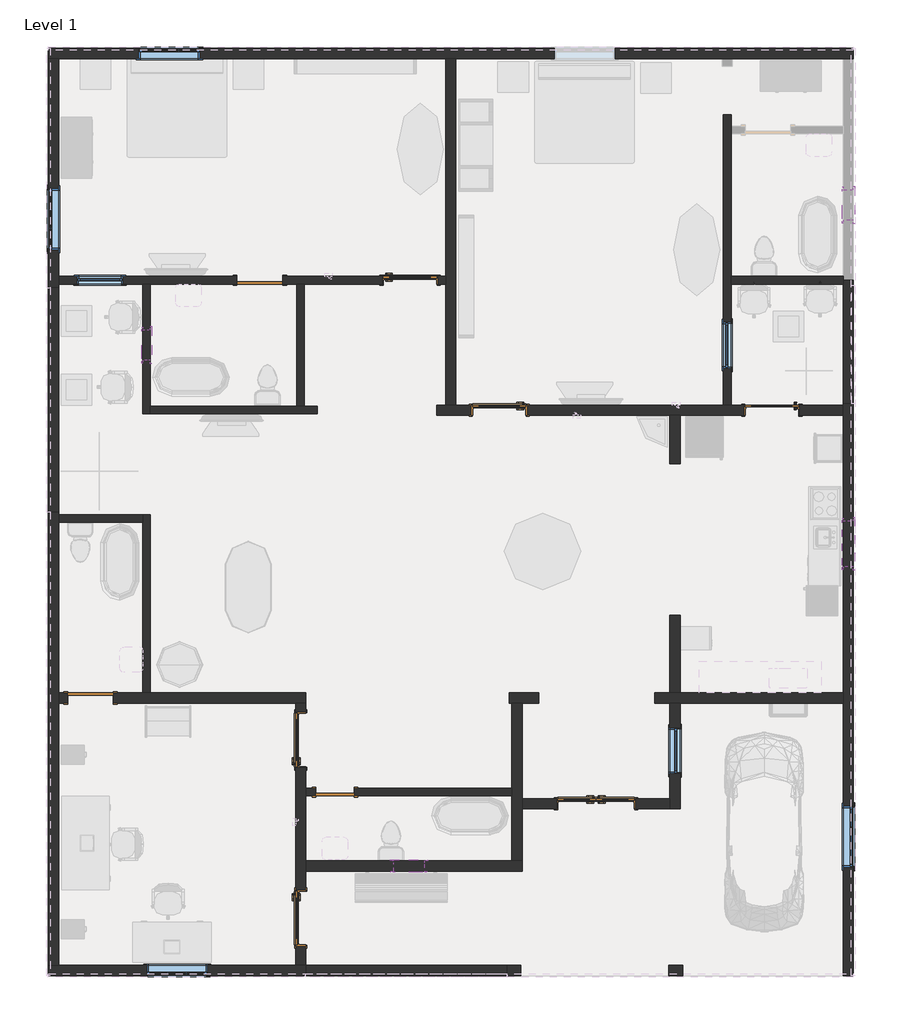
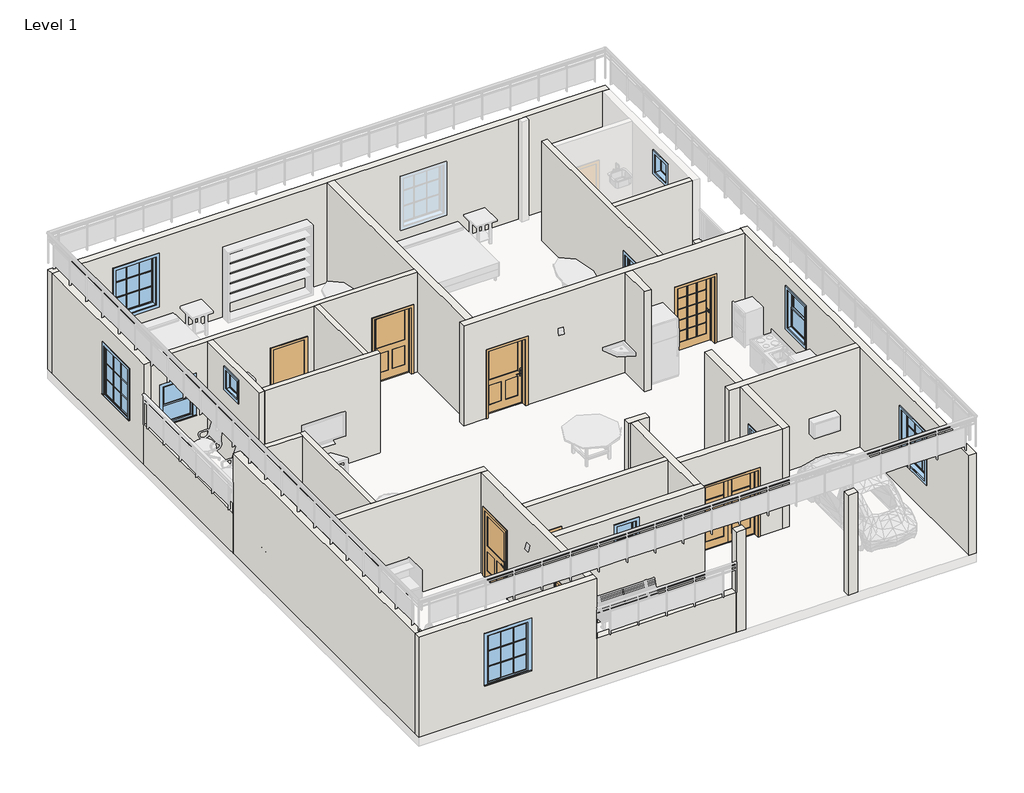
# One storey, part 1 of 4: 31 walls, 11 windows, 9 doors.
"""IFC4 building model written with IfcOpenShell, lengths in millimetres."""

from ifc_helpers import new_model, si_unit, frame, origin, origin_with_axes, place, context, project, spatial, polyline, outline, extrude, faceted_brep, transform, mapped, element, save
from components import door_374e07cf, door_e0076512, door_f970b2d0, door_b03bd389, door_1d83da25, door_059fdd7e, door_719f80de, door_686f89d2, window_cfa1ffdd, window_31198920, window_d24d93a6, window_3d781103, window_e41d21a6

model = new_model("IFC4")

# Units and contexts
model_context = context("Model", 3, world=origin())
ifc_project = project(units=[si_unit("LENGTHUNIT", "METRE", prefix="MILLI")], contexts=[model_context])

# Site, building, storey
site = spatial("IfcSite", under=ifc_project)
building = spatial("IfcBuilding", under=site)
storey = spatial("IfcBuildingStorey", under=building, Name="Level 1", Elevation=0.0)

# Doors
placement = place(None, origin())
door_shape = door_374e07cf(model_context)
element("IfcDoor", 1, ObjectType="42\" x 80\"", at=placement, inside=storey, context=model_context, shape_type="MappedRepresentation", body=[
    mapped(door_shape, transform((-12615.7234731, -1219.5557719, 0.0), x_axis=(0.0, -1.0, 0.0), y_axis=(1.0, 0.0, 0.0), z_axis=(0.0, 0.0, 1.0))),
])
door_2_shape = door_e0076512(model_context)
element("IfcDoor", 2, ObjectType="42\" x 80\"", at=placement, inside=storey, context=model_context, shape_type="MappedRepresentation", body=[
    mapped(door_2_shape, transform((-12615.7234731, -4775.5557719, 0.0), x_axis=(0.0, 1.0, 0.0), y_axis=(-1.0, 0.0, 0.0), z_axis=(0.0, 0.0, 1.0))),
])
element("IfcDoor", 3, ObjectType="42\" x 80\"", at=placement, inside=storey, context=model_context, shape_type="MappedRepresentation", body=[
    mapped(door_2_shape, transform((-8650.1484731, 5362.2192281, 0.0), x_axis=(1.0, 0.0, 0.0), y_axis=(0.0, 1.0, 0.0), z_axis=(0.0, 0.0, 1.0))),
])
door_3_shape = door_f970b2d0(model_context)
element("IfcDoor", 4, ObjectType="42\" x 80\"", at=placement, inside=storey, context=model_context, shape_type="MappedRepresentation", body=[
    mapped(door_3_shape, transform((-10428.1484731, 7953.0192281, 0.0), x_axis=(-1.0, 0.0, 0.0), y_axis=(0.0, -1.0, 0.0), z_axis=(0.0, 0.0, 1.0))),
])
door_4_shape = door_b03bd389(model_context)
element("IfcDoor", 5, ObjectType="Door-Exterior-Double-Full Glass-Wood_Clad : 60\" x 80\"", at=placement, inside=storey, context=model_context, shape_type="MappedRepresentation", body=[
    mapped(door_4_shape, transform((-6719.7484731, -2486.3807719, 0.0), x_axis=(1.0, 0.0, 0.0), y_axis=(0.0, 1.0, 0.0), z_axis=(0.0, 0.0, 1.0))),
])
door_5_shape = door_1d83da25(model_context)
element("IfcDoor", 6, ObjectType="Door-Interior-Single-Full Glass-Wood : 42\" x 80\"", at=placement, inside=storey, context=model_context, shape_type="MappedRepresentation", body=[
    mapped(door_5_shape, transform((-3214.5484731, 5362.2192281, 0.0), x_axis=(-1.0, 0.0, 0.0), y_axis=(0.0, -1.0, 0.0), z_axis=(0.0, 0.0, 1.0))),
])
door_6_shape = door_059fdd7e(model_context)
element("IfcDoor", 7, ObjectType="Single-Flush : 30\" x 80\"", at=placement, inside=storey, context=model_context, shape_type="MappedRepresentation", body=[
    mapped(door_6_shape, transform((-11926.7484731, -2260.9557719, 0.0), x_axis=(-1.0, 0.0, 0.0), y_axis=(0.0, -1.0, 0.0), z_axis=(0.0, 0.0, 1.0))),
])
door_7_shape = door_719f80de(model_context)
element("IfcDoor", 8, ObjectType="Single-Flush : 36\" x 84\"", at=placement, inside=storey, context=model_context, shape_type="MappedRepresentation", body=[
    mapped(door_7_shape, transform((-16803.5484731, -381.3557719, 0.0), x_axis=(-1.0, 0.0, 0.0), y_axis=(0.0, -1.0, 0.0), z_axis=(0.0, 0.0, 1.0))),
])
door_8_shape = door_686f89d2(model_context)
element("IfcDoor", 9, ObjectType="Single-Flush : 36\" x 84\"", at=placement, inside=storey, context=model_context, shape_type="MappedRepresentation", body=[
    mapped(door_8_shape, transform((-13425.3484731, 7949.8442281, 0.0), x_axis=(1.0, 0.0, 0.0), y_axis=(0.0, 1.0, 0.0), z_axis=(0.0, 0.0, 1.0))),
])

# Walls
element("IfcWall", 10, ObjectType="Generic - 8\"", at=placement, inside=storey, context=model_context, shape_type="Brep", body=[
    faceted_brep([(-17641.7484731, 12369.4442281, 0.0), (-17438.5484731, 12369.4442281, 0.0), (-9716.9484731, 12369.4442281, 0.0), (-9513.7484731, 12369.4442281, 0.0), (-4205.1484731, 12369.4442281, 0.0), (-4001.9484731, 12369.4442281, 0.0), (-1792.1484731, 12369.4442281, 0.0), (-1588.9484731, 12369.4442281, 0.0), (-1588.9484731, 12369.4442281, 3048.0), (-1792.1484731, 12369.4442281, 3048.0), (-4001.9484731, 12369.4442281, 3048.0), (-4205.1484731, 12369.4442281, 3048.0), (-9513.7484731, 12369.4442281, 3048.0), (-9716.9484731, 12369.4442281, 3048.0), (-17438.5484731, 12369.4442281, 3048.0), (-17641.7484731, 12369.4442281, 3048.0), (-14619.1484731, 12369.4442281, 2540.0), (-14619.1484731, 12369.4442281, 1016.0), (-15838.3484731, 12369.4442281, 1016.0), (-15838.3484731, 12369.4442281, 2540.0), (-6338.7484731, 12369.4442281, 2438.4), (-6338.7484731, 12369.4442281, 914.4), (-7557.9484731, 12369.4442281, 914.4), (-7557.9484731, 12369.4442281, 2438.4), (-17641.7484731, 12572.6442281, 0.0), (-17641.7484731, 12572.6442281, 3048.0), (-1588.9484731, 12572.6442281, 3048.0), (-1588.9484731, 12572.6442281, 0.0), (-14619.1484731, 12572.6442281, 2540.0), (-15838.3484731, 12572.6442281, 2540.0), (-15838.3484731, 12572.6442281, 1016.0), (-14619.1484731, 12572.6442281, 1016.0), (-6338.7484731, 12572.6442281, 2438.4), (-7557.9484731, 12572.6442281, 2438.4), (-7557.9484731, 12572.6442281, 914.4), (-6338.7484731, 12572.6442281, 914.4)], [[[0, 1, 2, 3, 4, 5, 6, 7, 8, 9, 10, 11, 12, 13, 14, 15], [16, 17, 18, 19], [20, 21, 22, 23]], [[24, 25, 26, 27], [28, 29, 30, 31], [32, 33, 34, 35]], [[7, 6, 5, 4, 3, 2, 1, 0, 24, 27]], [[8, 7, 27, 26]], [[0, 15, 25, 24]], [[17, 16, 28, 31]], [[18, 17, 31, 30]], [[19, 18, 30, 29]], [[16, 19, 29, 28]], [[21, 20, 32, 35]], [[22, 21, 35, 34]], [[23, 22, 34, 33]], [[20, 23, 33, 32]], [[15, 14, 13, 12, 11, 10, 9, 8, 26, 25]]]),
])
element("IfcWall", 11, ObjectType="Generic - 8\"", at=placement, inside=storey, context=model_context, shape_type="Brep", body=[
    faceted_brep([(-17438.5484731, -5715.3557719, 0.0), (-17438.5484731, -482.9557719, 0.0), (-17438.5484731, -279.7557719, 0.0), (-17438.5484731, 3123.8442281, 0.0), (-17438.5484731, 3276.2442281, 0.0), (-17438.5484731, 3327.0442281, 0.0), (-17438.5484731, 3327.0442281, 1219.2), (-17438.5484731, 3327.0442281, 3048.0), (-17438.5484731, 3276.2442281, 3048.0), (-17438.5484731, 3123.8442281, 3048.0), (-17438.5484731, -279.7557719, 3048.0), (-17438.5484731, -482.9557719, 3048.0), (-17438.5484731, -5715.3557719, 3048.0), (-17641.7484731, -5715.3557719, 0.0), (-17641.7484731, -5715.3557719, 3048.0), (-17641.7484731, 3327.0442281, 3048.0), (-17641.7484731, 3327.0442281, 1219.2), (-17641.7484731, 3327.0442281, 0.0)], [[[0, 1, 2, 3, 4, 5, 6, 7, 8, 9, 10, 11, 12]], [[13, 14, 15, 16, 17]], [[5, 4, 3, 2, 1, 0, 13, 17]], [[7, 6, 5, 17, 16, 15]], [[0, 12, 14, 13]], [[12, 11, 10, 9, 8, 7, 15, 14]]]),
])
element("IfcWall", 12, ObjectType="Generic - 8\"", at=placement, inside=storey, context=model_context, shape_type="Brep", body=[
    faceted_brep([(-9716.9484731, 12369.4442281, 0.0), (-9716.9484731, 8026.0442281, 0.0), (-9716.9484731, 7873.6442281, 0.0), (-9716.9484731, 5460.6442281, 0.0), (-9716.9484731, 5460.6442281, 3048.0), (-9716.9484731, 7873.6442281, 3048.0), (-9716.9484731, 8026.0442281, 3048.0), (-9716.9484731, 12369.4442281, 3048.0), (-9513.7484731, 12369.4442281, 0.0), (-9513.7484731, 12369.4442281, 3048.0), (-9513.7484731, 5460.6442281, 3048.0), (-9513.7484731, 5460.6442281, 0.0)], [[[0, 1, 2, 3, 4, 5, 6, 7]], [[8, 9, 10, 11]], [[3, 2, 1, 0, 8, 11]], [[0, 7, 9, 8]], [[4, 3, 11, 10]], [[7, 6, 5, 4, 10, 9]]]),
])
element("IfcWall", 13, ObjectType="Generic - 8\"", at=placement, inside=storey, context=model_context, shape_type="Brep", body=[
    faceted_brep([(-1792.1484731, -279.7557719, 0.0), (-5043.3484731, -279.7557719, 0.0), (-5246.5484731, -279.7557719, 0.0), (-5551.3484731, -279.7557719, 0.0), (-5551.3484731, -279.7557719, 3048.0), (-5246.5484731, -279.7557719, 3048.0), (-5043.3484731, -279.7557719, 3048.0), (-1792.1484731, -279.7557719, 3048.0), (-1792.1484731, -482.9557719, 0.0), (-1792.1484731, -482.9557719, 3048.0), (-5043.3484731, -482.9557719, 3048.0), (-5246.5484731, -482.9557719, 3048.0), (-5551.3484731, -482.9557719, 3048.0), (-5551.3484731, -482.9557719, 0.0), (-5246.5484731, -482.9557719, 0.0), (-5043.3484731, -482.9557719, 0.0)], [[[0, 1, 2, 3, 4, 5, 6, 7]], [[8, 9, 10, 11, 12, 13, 14, 15]], [[3, 2, 1, 0, 8, 15, 14, 13]], [[4, 3, 13, 12]], [[0, 7, 9, 8]], [[7, 6, 5, 4, 12, 11, 10, 9]]]),
])
element("IfcWall", 14, ObjectType="Generic - 8\"", at=placement, inside=storey, context=model_context, shape_type="Brep", body=[
    faceted_brep([(-12510.9484731, -3835.7557719, 0.0), (-8192.9484731, -3835.7557719, 0.0), (-8192.9484731, -3835.7557719, 3048.0), (-12510.9484731, -3835.7557719, 3048.0), (-10148.7484731, -3835.7557719, 2768.6), (-10148.7484731, -3835.7557719, 2159.0), (-10758.3484731, -3835.7557719, 2159.0), (-10758.3484731, -3835.7557719, 2768.6), (-12510.9484731, -3632.5557719, 0.0), (-12510.9484731, -3632.5557719, 3048.0), (-8396.1484731, -3632.5557719, 3048.0), (-8192.9484731, -3632.5557719, 3048.0), (-8192.9484731, -3632.5557719, 0.0), (-8396.1484731, -3632.5557719, 0.0), (-10148.7484731, -3632.5557719, 2768.6), (-10758.3484731, -3632.5557719, 2768.6), (-10758.3484731, -3632.5557719, 2159.0), (-10148.7484731, -3632.5557719, 2159.0)], [[[0, 1, 2, 3], [4, 5, 6, 7]], [[8, 9, 10, 11, 12, 13], [14, 15, 16, 17]], [[1, 0, 8, 13, 12]], [[0, 3, 9, 8]], [[2, 1, 12, 11]], [[3, 2, 11, 10, 9]], [[5, 4, 14, 17]], [[6, 5, 17, 16]], [[7, 6, 16, 15]], [[4, 7, 15, 14]]]),
])
element("IfcWall", 15, ObjectType="Generic - 8\"", at=placement, inside=storey, context=model_context, shape_type="Brep", body=[
    faceted_brep([(-8192.9484731, -3632.5557719, 0.0), (-8192.9484731, -2591.1557719, 0.0), (-8192.9484731, -2387.9557719, 0.0), (-8192.9484731, -482.9557719, 0.0), (-8192.9484731, -482.9557719, 3048.0), (-8192.9484731, -2387.9557719, 3048.0), (-8192.9484731, -2591.1557719, 3048.0), (-8192.9484731, -3632.5557719, 3048.0), (-8396.1484731, -3632.5557719, 0.0), (-8396.1484731, -3632.5557719, 3048.0), (-8396.1484731, -2337.1557719, 3048.0), (-8396.1484731, -2184.7557719, 3048.0), (-8396.1484731, -482.9557719, 3048.0), (-8396.1484731, -482.9557719, 0.0), (-8396.1484731, -2184.7557719, 0.0), (-8396.1484731, -2337.1557719, 0.0)], [[[0, 1, 2, 3, 4, 5, 6, 7]], [[8, 9, 10, 11, 12, 13, 14, 15]], [[3, 2, 1, 0, 8, 15, 14, 13]], [[0, 7, 9, 8]], [[4, 3, 13, 12]], [[7, 6, 5, 4, 12, 11, 10, 9]]]),
])
element("IfcWall", 16, ObjectType="Generic - 8\"", at=placement, inside=storey, context=model_context, shape_type="Brep", body=[
    faceted_brep([(-5246.5484731, -482.9557719, 0.0), (-5246.5484731, -2387.9557719, 0.0), (-5246.5484731, -2591.1557719, 0.0), (-5246.5484731, -2591.1557719, 3048.0), (-5246.5484731, -2387.9557719, 3048.0), (-5246.5484731, -482.9557719, 3048.0), (-5246.5484731, -1892.6557719, 2133.6), (-5246.5484731, -1892.6557719, 914.4), (-5246.5484731, -978.2557719, 914.4), (-5246.5484731, -978.2557719, 2133.6), (-5043.3484731, -482.9557719, 0.0), (-5043.3484731, -482.9557719, 3048.0), (-5043.3484731, -2591.1557719, 3048.0), (-5043.3484731, -2591.1557719, 0.0), (-5043.3484731, -1892.6557719, 2133.6), (-5043.3484731, -978.2557719, 2133.6), (-5043.3484731, -978.2557719, 914.4), (-5043.3484731, -1892.6557719, 914.4)], [[[0, 1, 2, 3, 4, 5], [6, 7, 8, 9]], [[10, 11, 12, 13], [14, 15, 16, 17]], [[2, 1, 0, 10, 13]], [[0, 5, 11, 10]], [[3, 2, 13, 12]], [[7, 6, 14, 17]], [[8, 7, 17, 16]], [[9, 8, 16, 15]], [[6, 9, 15, 14]], [[5, 4, 3, 12, 11]]]),
])
element("IfcWall", 17, ObjectType="Generic - 8\"", at=placement, inside=storey, context=model_context, shape_type="SweptSolid", body=[
    extrude(outline(polyline([(0.0, -5246.5484731), (3048.0, -5246.5484731), (3048.0, -8192.9484731), (0.0, -8192.9484731), (0.0, -7507.1484731), (2057.4, -7507.1484731), (2057.4, -5932.3484731), (0.0, -5932.3484731), (0.0, -5246.5484731)])), frame((0.0, -2591.1557719, 0.0), z_axis=(0.0, 1.0, 0.0), x_axis=(0.0, 0.0, 1.0)), (0.0, 0.0, 1.0), 203.2),
])
element("IfcWall", 18, ObjectType="Generic - 8\"", at=placement, inside=storey, context=model_context, shape_type="SweptSolid", body=[
    extrude(outline(polyline([(-5043.3484731, 1269.6442281), (-5043.3484731, -279.7557719), (-5246.5484731, -279.7557719), (-5246.5484731, 1269.6442281), (-5043.3484731, 1269.6442281)])), origin_with_axes(), (0.0, 0.0, 1.0), 3048.0),
])
element("IfcWall", 19, ObjectType="Generic - 8\"", at=placement, inside=storey, context=model_context, shape_type="Brep", body=[
    faceted_brep([(-9894.7484731, 5257.4442281, 3048.0), (-9894.7484731, 5257.4442281, 0.0), (-9208.9484731, 5257.4442281, 0.0), (-9208.9484731, 5257.4442281, 2057.4), (-8091.3484731, 5257.4442281, 2057.4), (-8091.3484731, 5257.4442281, 0.0), (-5246.5484731, 5257.4442281, 0.0), (-5043.3484731, 5257.4442281, 0.0), (-3773.3484731, 5257.4442281, 0.0), (-3773.3484731, 5257.4442281, 2057.4), (-2655.7484731, 5257.4442281, 2057.4), (-2655.7484731, 5257.4442281, 0.0), (-1792.1484731, 5257.4442281, 0.0), (-1792.1484731, 5257.4442281, 3048.0), (-5043.3484731, 5257.4442281, 3048.0), (-5246.5484731, 5257.4442281, 3048.0), (-9894.7484731, 5460.6442281, 0.0), (-9894.7484731, 5460.6442281, 3048.0), (-9716.9484731, 5460.6442281, 3048.0), (-9513.7484731, 5460.6442281, 3048.0), (-4179.7484731, 5460.6442281, 3048.0), (-4027.3484731, 5460.6442281, 3048.0), (-1792.1484731, 5460.6442281, 3048.0), (-1792.1484731, 5460.6442281, 0.0), (-2655.7484731, 5460.6442281, 0.0), (-2655.7484731, 5460.6442281, 2057.4), (-3773.3484731, 5460.6442281, 2057.4), (-3773.3484731, 5460.6442281, 0.0), (-4027.3484731, 5460.6442281, 0.0), (-4179.7484731, 5460.6442281, 0.0), (-8091.3484731, 5460.6442281, 0.0), (-8091.3484731, 5460.6442281, 2057.4), (-9208.9484731, 5460.6442281, 2057.4), (-9208.9484731, 5460.6442281, 0.0), (-9513.7484731, 5460.6442281, 0.0), (-9716.9484731, 5460.6442281, 0.0)], [[[0, 1, 2, 3, 4, 5, 6, 7, 8, 9, 10, 11, 12, 13, 14, 15]], [[16, 17, 18, 19, 20, 21, 22, 23, 24, 25, 26, 27, 28, 29, 30, 31, 32, 33, 34, 35]], [[1, 16, 35, 34, 33, 2]], [[23, 12, 11, 24]], [[5, 30, 29, 28, 27, 8, 7, 6]], [[1, 0, 17, 16]], [[13, 12, 23, 22]], [[4, 31, 30, 5]], [[31, 4, 3, 32]], [[32, 3, 2, 33]], [[26, 9, 8, 27]], [[9, 26, 25, 10]], [[10, 25, 24, 11]], [[0, 15, 14, 13, 22, 21, 20, 19, 18, 17]]]),
])
element("IfcWall", 20, ObjectType="Generic - 8\"", at=placement, inside=storey, context=model_context, shape_type="Brep", body=[
    faceted_brep([(-12714.1484731, -482.9557719, 3048.0), (-12714.1484731, -482.9557719, 0.0), (-12714.1484731, -660.7557719, 0.0), (-12714.1484731, -660.7557719, 2057.4), (-12714.1484731, -1778.3557719, 2057.4), (-12714.1484731, -1778.3557719, 0.0), (-12714.1484731, -4216.7557719, 0.0), (-12714.1484731, -4216.7557719, 2057.4), (-12714.1484731, -5334.3557719, 2057.4), (-12714.1484731, -5334.3557719, 0.0), (-12714.1484731, -5715.3557719, 0.0), (-12714.1484731, -5715.3557719, 3048.0), (-12510.9484731, -482.9557719, 0.0), (-12510.9484731, -482.9557719, 3048.0), (-12510.9484731, -2184.7557719, 3048.0), (-12510.9484731, -2337.1557719, 3048.0), (-12510.9484731, -3632.5557719, 3048.0), (-12510.9484731, -3835.7557719, 3048.0), (-12510.9484731, -5715.3557719, 3048.0), (-12510.9484731, -5715.3557719, 0.0), (-12510.9484731, -5334.3557719, 0.0), (-12510.9484731, -5334.3557719, 2057.4), (-12510.9484731, -4216.7557719, 2057.4), (-12510.9484731, -4216.7557719, 0.0), (-12510.9484731, -3835.7557719, 0.0), (-12510.9484731, -3632.5557719, 0.0), (-12510.9484731, -2337.1557719, 0.0), (-12510.9484731, -2184.7557719, 0.0), (-12510.9484731, -1778.3557719, 0.0), (-12510.9484731, -1778.3557719, 2057.4), (-12510.9484731, -660.7557719, 2057.4), (-12510.9484731, -660.7557719, 0.0)], [[[0, 1, 2, 3, 4, 5, 6, 7, 8, 9, 10, 11]], [[12, 13, 14, 15, 16, 17, 18, 19, 20, 21, 22, 23, 24, 25, 26, 27, 28, 29, 30, 31]], [[19, 10, 9, 20]], [[1, 12, 31, 2]], [[5, 28, 27, 26, 25, 24, 23, 6]], [[1, 0, 13, 12]], [[10, 19, 18, 11]], [[4, 29, 28, 5]], [[29, 4, 3, 30]], [[30, 3, 2, 31]], [[22, 7, 6, 23]], [[7, 22, 21, 8]], [[8, 21, 20, 9]], [[0, 11, 18, 17, 16, 15, 14, 13]]]),
])
element("IfcWall", 21, ObjectType="Generic - 8\"", at=placement, inside=storey, context=model_context, shape_type="Brep", body=[
    faceted_brep([(-12510.9484731, -5715.3557719, 0.0), (-12714.1484731, -5715.3557719, 0.0), (-17438.5484731, -5715.3557719, 0.0), (-17641.7484731, -5715.3557719, 0.0), (-17641.7484731, -5715.3557719, 3048.0), (-17438.5484731, -5715.3557719, 3048.0), (-12714.1484731, -5715.3557719, 3048.0), (-12510.9484731, -5715.3557719, 3048.0), (-12510.9484731, -5715.3557719, 1219.2), (-15685.9484731, -5715.3557719, 2438.4), (-15685.9484731, -5715.3557719, 914.4), (-14466.7484731, -5715.3557719, 914.4), (-14466.7484731, -5715.3557719, 2438.4), (-12510.9484731, -5918.5557719, 0.0), (-12510.9484731, -5918.5557719, 1219.2), (-12510.9484731, -5918.5557719, 3048.0), (-17641.7484731, -5918.5557719, 3048.0), (-17641.7484731, -5918.5557719, 0.0), (-15685.9484731, -5918.5557719, 2438.4), (-14466.7484731, -5918.5557719, 2438.4), (-14466.7484731, -5918.5557719, 914.4), (-15685.9484731, -5918.5557719, 914.4)], [[[0, 1, 2, 3, 4, 5, 6, 7, 8], [9, 10, 11, 12]], [[13, 14, 15, 16, 17], [18, 19, 20, 21]], [[3, 2, 1, 0, 13, 17]], [[0, 8, 7, 15, 14, 13]], [[4, 3, 17, 16]], [[10, 9, 18, 21]], [[11, 10, 21, 20]], [[12, 11, 20, 19]], [[9, 12, 19, 18]], [[7, 6, 5, 4, 16, 15]]]),
])
element("IfcWall", 22, ObjectType="Generic - 8\"", at=placement, inside=storey, context=model_context, shape_type="SweptSolid", body=[
    extrude(outline(polyline([(-12510.9484731, -5715.3557719), (-8497.7484731, -5715.3557719), (-8497.7484731, -5918.5557719), (-12510.9484731, -5918.5557719), (-12510.9484731, -5715.3557719)])), origin_with_axes(), (0.0, 0.0, 1.0), 1219.2),
])
element("IfcWall", 23, ObjectType="Generic - 8\"", at=placement, inside=storey, context=model_context, shape_type="Brep", body=[
    faceted_brep([(-8218.3484731, -5715.3557719, 0.0), (-8497.7484731, -5715.3557719, 0.0), (-8497.7484731, -5715.3557719, 1219.2), (-8497.7484731, -5715.3557719, 3048.0), (-8218.3484731, -5715.3557719, 3048.0), (-8218.3484731, -5918.5557719, 0.0), (-8218.3484731, -5918.5557719, 3048.0), (-8497.7484731, -5918.5557719, 3048.0), (-8497.7484731, -5918.5557719, 1219.2), (-8497.7484731, -5918.5557719, 0.0)], [[[0, 1, 2, 3, 4]], [[5, 6, 7, 8, 9]], [[1, 0, 5, 9]], [[3, 2, 1, 9, 8, 7]], [[0, 4, 6, 5]], [[4, 3, 7, 6]]]),
])
element("IfcWall", 24, ObjectType="Generic - 8\"", at=placement, inside=storey, context=model_context, shape_type="SweptSolid", body=[
    extrude(outline(polyline([(-5271.9484731, -5715.3557719), (-4992.5484731, -5715.3557719), (-4992.5484731, -5918.5557719), (-5271.9484731, -5918.5557719), (-5271.9484731, -5715.3557719)])), origin_with_axes(), (0.0, 0.0, 1.0), 3048.0),
])
element("IfcWall", 25, ObjectType="Generic - 8\"", at=placement, inside=storey, context=model_context, shape_type="Brep", body=[
    faceted_brep([(-17438.5484731, 7797.4442281, 0.0), (-17438.5484731, 7873.6442281, 0.0), (-17438.5484731, 8026.0442281, 0.0), (-17438.5484731, 12369.4442281, 0.0), (-17438.5484731, 12369.4442281, 3048.0), (-17438.5484731, 8026.0442281, 3048.0), (-17438.5484731, 7873.6442281, 3048.0), (-17438.5484731, 7797.4442281, 3048.0), (-17438.5484731, 7797.4442281, 1219.2), (-17438.5484731, 9778.6442281, 2438.4), (-17438.5484731, 9778.6442281, 914.4), (-17438.5484731, 8559.4442281, 914.4), (-17438.5484731, 8559.4442281, 2438.4), (-17641.7484731, 7797.4442281, 0.0), (-17641.7484731, 7797.4442281, 1219.2), (-17641.7484731, 7797.4442281, 3048.0), (-17641.7484731, 12369.4442281, 3048.0), (-17641.7484731, 12369.4442281, 0.0), (-17641.7484731, 9778.6442281, 2438.4), (-17641.7484731, 8559.4442281, 2438.4), (-17641.7484731, 8559.4442281, 914.4), (-17641.7484731, 9778.6442281, 914.4)], [[[0, 1, 2, 3, 4, 5, 6, 7, 8], [9, 10, 11, 12]], [[13, 14, 15, 16, 17], [18, 19, 20, 21]], [[3, 2, 1, 0, 13, 17]], [[0, 8, 7, 15, 14, 13]], [[4, 3, 17, 16]], [[10, 9, 18, 21]], [[11, 10, 21, 20]], [[12, 11, 20, 19]], [[9, 12, 19, 18]], [[7, 6, 5, 4, 16, 15]]]),
])
element("IfcWall", 26, ObjectType="Generic - 8\"", at=placement, inside=storey, context=model_context, shape_type="SweptSolid", body=[
    extrude(outline(polyline([(-17438.5484731, 7797.4442281), (-17438.5484731, 3327.0442281), (-17641.7484731, 3327.0442281), (-17641.7484731, 7797.4442281), (-17438.5484731, 7797.4442281)])), origin_with_axes(), (0.0, 0.0, 1.0), 1219.2),
])
element("IfcWall", 27, ObjectType="Generic - 8\"", at=placement, inside=storey, context=model_context, shape_type="Brep", body=[
    faceted_brep([(-17260.7484731, -279.7557719, 2133.6), (-17260.7484731, -279.7557719, 0.0), (-17438.5484731, -279.7557719, 0.0), (-17438.5484731, -279.7557719, 3048.0), (-15762.1484731, -279.7557719, 3048.0), (-15609.7484731, -279.7557719, 3048.0), (-12510.9484731, -279.7557719, 3048.0), (-12510.9484731, -279.7557719, 0.0), (-15609.7484731, -279.7557719, 0.0), (-15762.1484731, -279.7557719, 0.0), (-16346.3484731, -279.7557719, 0.0), (-16346.3484731, -279.7557719, 2133.6), (-17438.5484731, -482.9557719, 0.0), (-17260.7484731, -482.9557719, 0.0), (-17260.7484731, -482.9557719, 2133.6), (-16346.3484731, -482.9557719, 2133.6), (-16346.3484731, -482.9557719, 0.0), (-12714.1484731, -482.9557719, 0.0), (-12510.9484731, -482.9557719, 0.0), (-12510.9484731, -482.9557719, 3048.0), (-12714.1484731, -482.9557719, 3048.0), (-17438.5484731, -482.9557719, 3048.0)], [[[0, 1, 2, 3, 4, 5, 6, 7, 8, 9, 10, 11]], [[12, 13, 14, 15, 16, 17, 18, 19, 20, 21]], [[2, 1, 13, 12]], [[10, 9, 8, 7, 18, 17, 16]], [[7, 6, 19, 18]], [[3, 2, 12, 21]], [[14, 13, 1, 0]], [[15, 14, 0, 11]], [[16, 15, 11, 10]], [[6, 5, 4, 3, 21, 20, 19]]]),
])
element("IfcWall", 28, ObjectType="Generic - 8\"", at=placement, inside=storey, context=model_context, shape_type="Brep", body=[
    faceted_brep([(-7862.7484731, -279.7557719, 0.0), (-8446.9484731, -279.7557719, 0.0), (-8446.9484731, -279.7557719, 3048.0), (-7862.7484731, -279.7557719, 3048.0), (-7862.7484731, -482.9557719, 0.0), (-7862.7484731, -482.9557719, 3048.0), (-8192.9484731, -482.9557719, 3048.0), (-8396.1484731, -482.9557719, 3048.0), (-8446.9484731, -482.9557719, 3048.0), (-8446.9484731, -482.9557719, 0.0), (-8396.1484731, -482.9557719, 0.0), (-8192.9484731, -482.9557719, 0.0)], [[[0, 1, 2, 3]], [[4, 5, 6, 7, 8, 9, 10, 11]], [[1, 0, 4, 11, 10, 9]], [[2, 1, 9, 8]], [[0, 3, 5, 4]], [[3, 2, 8, 7, 6, 5]]]),
])
element("IfcWall", 29, ObjectType="Generic - 8\"", at=placement, inside=storey, context=model_context, shape_type="SweptSolid", body=[
    extrude(outline(polyline([(-5043.3484731, 5257.4442281), (-5043.3484731, 4292.2442281), (-5246.5484731, 4292.2442281), (-5246.5484731, 5257.4442281), (-5043.3484731, 5257.4442281)])), origin_with_axes(), (0.0, 0.0, 1.0), 3048.0),
])
element("IfcWall", 30, ObjectType="Generic - 8\"", at=placement, inside=storey, context=model_context, shape_type="Brep", body=[
    faceted_brep([(-1792.1484731, 7949.8442281, 0.0), (-1792.1484731, 7873.6442281, 0.0), (-1792.1484731, 5486.0442281, 0.0), (-1792.1484731, 5486.0442281, 1219.2), (-1792.1484731, 7873.6442281, 1219.2), (-1792.1484731, 7949.8442281, 1219.2), (-1588.9484731, 7949.8442281, 0.0), (-1588.9484731, 7949.8442281, 1219.2), (-1588.9484731, 7873.6442281, 1219.2), (-1588.9484731, 5486.0442281, 1219.2), (-1588.9484731, 5486.0442281, 0.0)], [[[0, 1, 2, 3, 4, 5]], [[6, 7, 8, 9, 10]], [[2, 1, 0, 6, 10]], [[3, 2, 10, 9]], [[5, 4, 3, 9, 8, 7]], [[0, 5, 7, 6]]]),
])
element("IfcWall", 31, ObjectType="Generic - 8\"", at=placement, inside=storey, context=model_context, shape_type="Brep", body=[
    faceted_brep([(-1792.1484731, 5486.0442281, 0.0), (-1792.1484731, 5460.6442281, 0.0), (-1792.1484731, 5257.4442281, 0.0), (-1792.1484731, -279.7557719, 0.0), (-1792.1484731, -482.9557719, 0.0), (-1792.1484731, -5918.5557719, 0.0), (-1792.1484731, -5918.5557719, 3048.0), (-1792.1484731, -482.9557719, 3048.0), (-1792.1484731, -279.7557719, 3048.0), (-1792.1484731, 5257.4442281, 3048.0), (-1792.1484731, 5460.6442281, 3048.0), (-1792.1484731, 5486.0442281, 3048.0), (-1792.1484731, 5486.0442281, 1219.2), (-1792.1484731, -3759.5557719, 2438.4), (-1792.1484731, -3759.5557719, 914.4), (-1792.1484731, -2540.3557719, 914.4), (-1792.1484731, -2540.3557719, 2438.4), (-1792.1484731, 2234.8442281, 2641.6), (-1792.1484731, 2234.8442281, 1422.4), (-1792.1484731, 3149.2442281, 1422.4), (-1792.1484731, 3149.2442281, 2641.6), (-1588.9484731, 5486.0442281, 0.0), (-1588.9484731, 5486.0442281, 1219.2), (-1588.9484731, 5486.0442281, 3048.0), (-1588.9484731, -5918.5557719, 3048.0), (-1588.9484731, -5918.5557719, 0.0), (-1588.9484731, -3759.5557719, 2438.4), (-1588.9484731, -2540.3557719, 2438.4), (-1588.9484731, -2540.3557719, 914.4), (-1588.9484731, -3759.5557719, 914.4), (-1588.9484731, 2234.8442281, 2641.6), (-1588.9484731, 3149.2442281, 2641.6), (-1588.9484731, 3149.2442281, 1422.4), (-1588.9484731, 2234.8442281, 1422.4)], [[[0, 1, 2, 3, 4, 5, 6, 7, 8, 9, 10, 11, 12], [13, 14, 15, 16], [17, 18, 19, 20]], [[21, 22, 23, 24, 25], [26, 27, 28, 29], [30, 31, 32, 33]], [[5, 4, 3, 2, 1, 0, 21, 25]], [[6, 5, 25, 24]], [[0, 12, 11, 23, 22, 21]], [[14, 13, 26, 29]], [[15, 14, 29, 28]], [[16, 15, 28, 27]], [[13, 16, 27, 26]], [[18, 17, 30, 33]], [[19, 18, 33, 32]], [[20, 19, 32, 31]], [[17, 20, 31, 30]], [[11, 10, 9, 8, 7, 6, 24, 23]]]),
])
element("IfcWall", 32, ObjectType="inner wall", at=placement, inside=storey, context=model_context, shape_type="Brep", body=[
    faceted_brep([(-17438.5484731, 8026.0442281, 0.0), (-17438.5484731, 8026.0442281, 3048.0), (-9716.9484731, 8026.0442281, 3048.0), (-9716.9484731, 8026.0442281, 0.0), (-9869.3484731, 8026.0442281, 0.0), (-9869.3484731, 8026.0442281, 2057.4), (-10986.9484731, 8026.0442281, 2057.4), (-10986.9484731, 8026.0442281, 0.0), (-12968.1484731, 8026.0442281, 0.0), (-12968.1484731, 8026.0442281, 2133.6), (-13882.5484731, 8026.0442281, 2133.6), (-13882.5484731, 8026.0442281, 0.0), (-17070.2484731, 8026.0442281, 2133.6), (-17070.2484731, 8026.0442281, 914.4), (-16155.8484731, 8026.0442281, 914.4), (-16155.8484731, 8026.0442281, 2133.6), (-17438.5484731, 7873.6442281, 3048.0), (-17438.5484731, 7873.6442281, 0.0), (-15762.1484731, 7873.6442281, 0.0), (-15609.7484731, 7873.6442281, 0.0), (-13882.5484731, 7873.6442281, 0.0), (-13882.5484731, 7873.6442281, 2133.6), (-12968.1484731, 7873.6442281, 2133.6), (-12968.1484731, 7873.6442281, 0.0), (-12688.7484731, 7873.6442281, 0.0), (-12536.3484731, 7873.6442281, 0.0), (-10986.9484731, 7873.6442281, 0.0), (-10986.9484731, 7873.6442281, 2057.4), (-9869.3484731, 7873.6442281, 2057.4), (-9869.3484731, 7873.6442281, 0.0), (-9716.9484731, 7873.6442281, 0.0), (-9716.9484731, 7873.6442281, 3048.0), (-12536.3484731, 7873.6442281, 3048.0), (-12688.7484731, 7873.6442281, 3048.0), (-15609.7484731, 7873.6442281, 3048.0), (-15762.1484731, 7873.6442281, 3048.0), (-17070.2484731, 7873.6442281, 2133.6), (-16155.8484731, 7873.6442281, 2133.6), (-16155.8484731, 7873.6442281, 914.4), (-17070.2484731, 7873.6442281, 914.4)], [[[0, 1, 2, 3, 4, 5, 6, 7, 8, 9, 10, 11], [12, 13, 14, 15]], [[16, 17, 18, 19, 20, 21, 22, 23, 24, 25, 26, 27, 28, 29, 30, 31, 32, 33, 34, 35], [36, 37, 38, 39]], [[3, 30, 29, 4]], [[17, 0, 11, 20, 19, 18]], [[23, 8, 7, 26, 25, 24]], [[1, 0, 17, 16]], [[3, 2, 31, 30]], [[9, 8, 23, 22]], [[10, 9, 22, 21]], [[11, 10, 21, 20]], [[6, 27, 26, 7]], [[27, 6, 5, 28]], [[28, 5, 4, 29]], [[13, 12, 36, 39]], [[14, 13, 39, 38]], [[15, 14, 38, 37]], [[12, 15, 37, 36]], [[2, 1, 16, 35, 34, 33, 32, 31]]]),
])
element("IfcWall", 33, ObjectType="inner wall", at=placement, inside=storey, context=model_context, shape_type="Brep", body=[
    faceted_brep([(-15762.1484731, 7873.6442281, 0.0), (-15762.1484731, 5282.8442281, 0.0), (-15762.1484731, 5282.8442281, 3048.0), (-15762.1484731, 7873.6442281, 3048.0), (-15762.1484731, 6349.6442281, 2768.6), (-15762.1484731, 6349.6442281, 2159.0), (-15762.1484731, 6959.2442281, 2159.0), (-15762.1484731, 6959.2442281, 2768.6), (-15609.7484731, 7873.6442281, 0.0), (-15609.7484731, 7873.6442281, 3048.0), (-15609.7484731, 5435.2442281, 3048.0), (-15609.7484731, 5282.8442281, 3048.0), (-15609.7484731, 5282.8442281, 0.0), (-15609.7484731, 5435.2442281, 0.0), (-15609.7484731, 6349.6442281, 2768.6), (-15609.7484731, 6959.2442281, 2768.6), (-15609.7484731, 6959.2442281, 2159.0), (-15609.7484731, 6349.6442281, 2159.0)], [[[0, 1, 2, 3], [4, 5, 6, 7]], [[8, 9, 10, 11, 12, 13], [14, 15, 16, 17]], [[1, 0, 8, 13, 12]], [[0, 3, 9, 8]], [[2, 1, 12, 11]], [[3, 2, 11, 10, 9]], [[5, 4, 14, 17]], [[6, 5, 17, 16]], [[7, 6, 16, 15]], [[4, 7, 15, 14]]]),
])
element("IfcWall", 34, ObjectType="inner wall", at=placement, inside=storey, context=model_context, shape_type="SweptSolid", body=[
    extrude(outline(polyline([(-17438.5484731, 3276.2442281), (-15762.1484731, 3276.2442281), (-15762.1484731, 3123.8442281), (-17438.5484731, 3123.8442281), (-17438.5484731, 3276.2442281)])), origin_with_axes(), (0.0, 0.0, 1.0), 3048.0),
])
element("IfcWall", 35, ObjectType="inner wall", at=placement, inside=storey, context=model_context, shape_type="SweptSolid", body=[
    extrude(outline(polyline([(-12688.7484731, 5435.2442281), (-12688.7484731, 7873.6442281), (-12536.3484731, 7873.6442281), (-12536.3484731, 5435.2442281), (-12688.7484731, 5435.2442281)])), origin_with_axes(), (0.0, 0.0, 1.0), 3048.0),
])
element("IfcWall", 36, ObjectType="inner wall", at=placement, inside=storey, context=model_context, shape_type="Brep", body=[
    faceted_brep([(-4027.3484731, 7873.6442281, 0.0), (-1792.1484731, 7873.6442281, 0.0), (-1792.1484731, 7873.6442281, 1219.2), (-1792.1484731, 7873.6442281, 3048.0), (-4027.3484731, 7873.6442281, 3048.0), (-4027.3484731, 8026.0442281, 0.0), (-4027.3484731, 8026.0442281, 3048.0), (-1792.1484731, 8026.0442281, 3048.0), (-1792.1484731, 8026.0442281, 0.0), (-1792.1484731, 7949.8442281, 0.0)], [[[0, 1, 2, 3, 4]], [[5, 6, 7, 8]], [[1, 0, 5, 8, 9]], [[0, 4, 6, 5]], [[1, 9, 8, 7, 3, 2]], [[4, 3, 7, 6]]]),
])
element("IfcWall", 37, ObjectType="inner wall", at=placement, inside=storey, context=model_context, shape_type="Brep", body=[
    faceted_brep([(-15762.1484731, 3276.2442281, 0.0), (-15762.1484731, 3123.8442281, 0.0), (-15762.1484731, -279.7557719, 0.0), (-15762.1484731, -279.7557719, 3048.0), (-15762.1484731, 3123.8442281, 3048.0), (-15762.1484731, 3276.2442281, 3048.0), (-15609.7484731, 3276.2442281, 0.0), (-15609.7484731, 3276.2442281, 3048.0), (-15609.7484731, -279.7557719, 3048.0), (-15609.7484731, -279.7557719, 0.0)], [[[0, 1, 2, 3, 4, 5]], [[6, 7, 8, 9]], [[2, 1, 0, 6, 9]], [[3, 2, 9, 8]], [[0, 5, 7, 6]], [[5, 4, 3, 8, 7]]]),
])
element("IfcWall", 38, ObjectType="inner wall", at=placement, inside=storey, context=model_context, shape_type="Brep", body=[
    faceted_brep([(-15609.7484731, 5282.8442281, 0.0), (-12282.3484731, 5282.8442281, 0.0), (-12282.3484731, 5282.8442281, 3048.0), (-15609.7484731, 5282.8442281, 3048.0), (-15609.7484731, 5435.2442281, 0.0), (-15609.7484731, 5435.2442281, 3048.0), (-12688.7484731, 5435.2442281, 3048.0), (-12536.3484731, 5435.2442281, 3048.0), (-12282.3484731, 5435.2442281, 3048.0), (-12282.3484731, 5435.2442281, 0.0), (-12536.3484731, 5435.2442281, 0.0), (-12688.7484731, 5435.2442281, 0.0)], [[[0, 1, 2, 3]], [[4, 5, 6, 7, 8, 9, 10, 11]], [[1, 0, 4, 11, 10, 9]], [[2, 1, 9, 8]], [[0, 3, 5, 4]], [[3, 2, 8, 7, 6, 5]]]),
])
element("IfcWall", 39, ObjectType="inner wall", at=placement, inside=storey, context=model_context, shape_type="Brep", body=[
    faceted_brep([(-4027.3484731, 5460.6442281, 0.0), (-4027.3484731, 7873.6442281, 0.0), (-4027.3484731, 8026.0442281, 0.0), (-4027.3484731, 10870.8442281, 0.0), (-4027.3484731, 11023.2442281, 0.0), (-4027.3484731, 11251.8442281, 0.0), (-4027.3484731, 11251.8442281, 3048.0), (-4027.3484731, 11023.2442281, 3048.0), (-4027.3484731, 10870.8442281, 3048.0), (-4027.3484731, 8026.0442281, 3048.0), (-4027.3484731, 7873.6442281, 3048.0), (-4027.3484731, 5460.6442281, 3048.0), (-4027.3484731, 6197.2442281, 2133.6), (-4027.3484731, 7111.6442281, 2133.6), (-4027.3484731, 7111.6442281, 914.4), (-4027.3484731, 6197.2442281, 914.4), (-4179.7484731, 5460.6442281, 0.0), (-4179.7484731, 5460.6442281, 3048.0), (-4179.7484731, 11251.8442281, 3048.0), (-4179.7484731, 11251.8442281, 0.0), (-4179.7484731, 6197.2442281, 2133.6), (-4179.7484731, 6197.2442281, 914.4), (-4179.7484731, 7111.6442281, 914.4), (-4179.7484731, 7111.6442281, 2133.6)], [[[0, 1, 2, 3, 4, 5, 6, 7, 8, 9, 10, 11], [12, 13, 14, 15]], [[16, 17, 18, 19], [20, 21, 22, 23]], [[5, 4, 3, 2, 1, 0, 16, 19]], [[6, 5, 19, 18]], [[0, 11, 17, 16]], [[21, 20, 12, 15]], [[22, 21, 15, 14]], [[23, 22, 14, 13]], [[20, 23, 13, 12]], [[11, 10, 9, 8, 7, 6, 18, 17]]]),
])
element("IfcWall", 40, ObjectType="inner wall", at=placement, inside=storey, context=model_context, shape_type="SweptSolid", body=[
    extrude(outline(polyline([(0.0, -12510.9484731), (0.0, -12307.7484731), (2032.0, -12307.7484731), (2032.0, -11545.7484731), (0.0, -11545.7484731), (0.0, -8396.1484731), (3048.0, -8396.1484731), (3048.0, -12510.9484731), (0.0, -12510.9484731)])), frame((0.0, -2337.1557719, 0.0), z_axis=(0.0, 1.0, 0.0), x_axis=(0.0, 0.0, 1.0)), (0.0, 0.0, 1.0), 152.4),
])

# Windows
window_shape = window_cfa1ffdd(model_context)
element("IfcWindow", 41, ObjectType="Casement 3x3 with Trim : 48\" x 60\"", at=placement, inside=storey, context=model_context, shape_type="MappedRepresentation", body=[
    mapped(window_shape, transform((-15076.3484731, -5816.9557719, 304.8), x_axis=(-1.0, 0.0, 0.0), y_axis=(0.0, -1.0, 0.0), z_axis=(0.0, 0.0, 1.0))),
])
element("IfcWindow", 42, ObjectType="Casement 3x3 with Trim : 48\" x 60\"", at=placement, inside=storey, context=model_context, shape_type="MappedRepresentation", body=[
    mapped(window_shape, transform((-15228.7484731, 12471.0442281, 406.4), x_axis=(1.0, 0.0, 0.0), y_axis=(0.0, 1.0, 0.0), z_axis=(0.0, 0.0, 1.0))),
])
element("IfcWindow", 43, ObjectType="Casement 3x3 with Trim : 48\" x 60\"", at=placement, inside=storey, context=model_context, shape_type="MappedRepresentation", body=[
    mapped(window_shape, transform((-17540.1484731, 9169.0442281, 304.8), x_axis=(0.0, 1.0, 0.0), y_axis=(-1.0, 0.0, 0.0), z_axis=(0.0, 0.0, 1.0))),
])
element("IfcWindow", 44, ObjectType="Casement 3x3 with Trim : 48\" x 60\"", at=placement, inside=storey, context=model_context, shape_type="MappedRepresentation", body=[
    mapped(window_shape, transform((-1690.5484731, -3149.9557719, 304.8), x_axis=(0.0, -1.0, 0.0), y_axis=(1.0, 0.0, 0.0), z_axis=(0.0, 0.0, 1.0))),
])
window_2_shape = window_31198920(model_context)
element("IfcWindow", 45, ObjectType="Double Hung with Trim : 36\" x 48\"", at=placement, inside=storey, context=model_context, shape_type="MappedRepresentation", body=[
    mapped(window_2_shape, transform((-1690.5484731, 2692.0442281, 508.0), x_axis=(0.0, -1.0, 0.0), y_axis=(1.0, 0.0, 0.0), z_axis=(0.0, 0.0, 1.0))),
])
element("IfcWindow", 46, ObjectType="Double Hung with Trim : 36\" x 48\"", at=placement, inside=storey, context=model_context, shape_type="MappedRepresentation", body=[
    mapped(window_2_shape, transform((-5144.9484731, -1435.4557719, 0.0), x_axis=(0.0, -1.0, 0.0), y_axis=(1.0, 0.0, 0.0), z_axis=(0.0, 0.0, 1.0))),
])
window_3_shape = window_d24d93a6(model_context)
element("IfcWindow", 47, ObjectType="Double Hung with Trim : 36\" x 48\"", at=placement, inside=storey, context=model_context, shape_type="MappedRepresentation", body=[
    mapped(window_3_shape, transform((-16613.0484731, 7949.8442281, 0.0), x_axis=(-1.0, 0.0, 0.0), y_axis=(0.0, -1.0, 0.0), z_axis=(0.0, 0.0, 1.0))),
])
element("IfcWindow", 48, ObjectType="Double Hung with Trim : 36\" x 48\"", at=placement, inside=storey, context=model_context, shape_type="MappedRepresentation", body=[
    mapped(window_3_shape, transform((-4103.5484731, 6654.4442281, 0.0), x_axis=(0.0, -1.0, 0.0), y_axis=(1.0, 0.0, 0.0), z_axis=(0.0, 0.0, 1.0))),
])
window_4_shape = window_3d781103(model_context)
element("IfcWindow", 49, ObjectType="Transom with Trim : 24\" x 24\"", at=placement, inside=storey, context=model_context, shape_type="MappedRepresentation", body=[
    mapped(window_4_shape, transform((-15685.9484731, 6616.3442281, 0.0), x_axis=(0.0, -1.0, 0.0), y_axis=(1.0, 0.0, 0.0), z_axis=(0.0, 0.0, 1.0))),
])
window_5_shape = window_e41d21a6(model_context)
element("IfcWindow", 50, ObjectType="Transom with Trim : 24\" x 24\"", at=placement, inside=storey, context=model_context, shape_type="MappedRepresentation", body=[
    mapped(window_5_shape, transform((-1690.5484731, 9410.3442281, 0.0), x_axis=(0.0, -1.0, 0.0), y_axis=(1.0, 0.0, 0.0), z_axis=(0.0, 0.0, 1.0))),
])
element("IfcWindow", 51, ObjectType="Transom with Trim : 24\" x 24\"", at=placement, inside=storey, context=model_context, shape_type="MappedRepresentation", body=[
    mapped(window_5_shape, transform((-10415.4484731, -3734.1557719, 0.0), x_axis=(1.0, 0.0, 0.0), y_axis=(0.0, 1.0, 0.0), z_axis=(0.0, 0.0, 1.0))),
])

save(model, "model.ifc")

# Revit data of these elements
# Type "42\" x 80\""
#   Type Mark = "9"
#   Assembly Code = "B2030100"
#   Analytic Construction = "French door, wood frame with single glass"
#   Top Rail = 0' - 4 3/4"
#   Threshold Offset [instance default] = 0' - 0 1/2"
#   Thickness = 0' - 1 3/8"
#   Thermal Resistance (R) = 1.0696 (h·ft²·°F)/BTU
#   Swing Angle [instance default] = 90.00°
#   Stiles = 0' - 4 3/4"
#   Rough Width = 3' - 8"
#   Rough Height = 6' - 9"
#   Lock Rail = 0' - 7 1/8"
#   Height = 6' - 8"
#   Width = 3' - 6"
#   Heat Transfer Coefficient (U) = 0.9350 BTU/(h·ft²·°F)
#   Door Offset [instance default] = 0' - 0"
#   Bottom Rail = 0' - 9 1/2"
#   Threshold [instance default] = yes
#   Function = 1
#   Exterior Trim [instance default] = yes
#   Trim Material = Cherry
#   Threshold Material = Cherry
#   Panel Material = Cherry
#   Glazing = Glass
#   Frame Material = Cherry
#   Door Handle Material = Aluminum
#   Visual Light Transmittance = 0
#   Solar Heat Gain Coefficient = 0
#   Wall Closure = (empty or 0)
#   Construction Type = (empty or 0)
# Type "Door-Exterior-Double-Full Glass-Wood_Clad : 60\" x 80\""
#   Type Mark = "8"
#   Assembly Code = "B2030100"
#   Analytic Construction = "French door, wood frame with double glass"
#   Top Rail = 0' - 4 11/16"
#   Threshold Offset [instance default] = 0' - 0 1/2"
#   Thickness = 0' - 1 3/8"
#   Thermal Resistance (R) = 1.9158 (h·ft²·°F)/BTU
#   Swing Angle [instance default] = 90.00°
#   Stiles = 0' - 4 3/4"
#   Rough Width = 5' - 2"
#   Rough Height = 6' - 9"
#   Panel Width = 2' - 6"
#   Door Offset [instance default] = 0' - 0"
#   Height = 6' - 8"
#   Width = 5' - 0"
#   Heat Transfer Coefficient (U) = 0.5220 BTU/(h·ft²·°F)
#   Bottom Rail = 0' - 9 1/8"
#   Exterior Trim [instance default] = yes
#   Threshold [instance default] = yes
#   Show Grill [instance default] = yes
#   Function = 1
#   Trim Material = Cherry
#   Threshold Material = Cherry
#   Panel Material = Cherry
#   Glazing = Glass
#   Frame Material = Cherry
#   Door Handle Material = Aluminum
#   Visual Light Transmittance = 0
#   Solar Heat Gain Coefficient = 0
#   Wall Closure = (empty or 0)
#   Construction Type = (empty or 0)
# Type "Door-Interior-Single-Full Glass-Wood : 42\" x 80\""
#   Type Mark = "10"
#   Assembly Code = "C1020300"
#   Analytic Construction = "Wood frame with single clear glass"
#   Top Rail = 0' - 4 11/16"
#   Thickness = 0' - 1 3/8"
#   Thermal Resistance (R) = 1.0102 (h·ft²·°F)/BTU
#   Swing Angle [instance default] = 90.00°
#   Stiles = 0' - 4 3/4"
#   Rough Width = 3' - 8"
#   Rough Height = 6' - 9"
#   Height = 6' - 8"
#   Width = 3' - 6"
#   Heat Transfer Coefficient (U) = 0.9900 BTU/(h·ft²·°F)
#   Bottom Rail = 0' - 9 1/8"
#   Show Grill [instance default] = yes
#   Trim Material = Cherry
#   Panel Material = Cherry
#   Frame Material = Cherry
#   Door Handle Material = Aluminum
#   Visual Light Transmittance = 0
#   Solar Heat Gain Coefficient = 0
#   Wall Closure = (empty or 0)
#   Function = (empty or 0)
# Type "Single-Flush : 30\" x 80\""
#   Type Mark = "5"
#   Construction Type Id = "MDOOR"
#   Assembly Code = "C1020"
#   Analytic Construction = "Metal"
#   Thickness = 0' - 2"
#   Heat Transfer Coefficient (U) = 0.651978 BTU/(h·ft²·°F)
#   Height = 6' - 8"
#   Trim Projection Ext = 0' - 1"
#   Trim Projection Int = 0' - 1"
#   Trim Width = 0' - 3"
#   Width = 2' - 6"
#   Define Thermal Properties by = 1
#   Door Material = Door - Panel
#   Frame Material = Door - Frame
#   Visual Light Transmittance = 0
#   Solar Heat Gain Coefficient = 0
#   Function = (empty or 0)
#   Wall Closure = (empty or 0)
# Type "Single-Flush : 36\" x 84\""
#   Type Mark = "1"
#   Construction Type Id = "MDOOR"
#   Assembly Code = "C1020"
#   Analytic Construction = "Metal"
#   Thickness = 0' - 2"
#   Heat Transfer Coefficient (U) = 0.651978 BTU/(h·ft²·°F)
#   Height = 7' - 0"
#   Trim Projection Ext = 0' - 1"
#   Trim Projection Int = 0' - 1"
#   Trim Width = 0' - 3"
#   Width = 3' - 0"
#   Define Thermal Properties by = 1
#   Door Material = Door - Panel
#   Frame Material = Door - Frame
#   Visual Light Transmittance = 0
#   Solar Heat Gain Coefficient = 0
#   Function = (empty or 0)
#   Wall Closure = (empty or 0)
# Type "Generic - 8\""
#   Assembly Code = "B2010"
#   Layers, outside or top first: 0' - 8" "Brick, Common" (function 1)
# Type "inner wall"
#   Assembly Code = "B2010"
#   Layers, outside or top first: 0' - 6" "Brick, Soldier Course" (function 1)
# Type "Casement 3x3 with Trim : 48\" x 60\""
#   Type Mark = "11"
#   Construction Type Id = "GSP4R"
#   Assembly Code = "B2020100"
#   Analytic Construction = "1/8 in Pilkington single glazing"
#   Visual Light Transmittance = 0.9
#   Solar Heat Gain Coefficient = 0.78
#   Heat Transfer Coefficient (U) = 0.6496 BTU/(h·ft²·°F)
#   Height = 5' - 0"
#   Default Sill Height = 2' - 0"
#   Trim Projection - Ext. = 0' - 0 1/2"
#   Trim Projection - Int. = 0' - 0 3/4"
#   Trim Width - Exterior = 0' - 3 1/2"
#   Trim Width - Interior = 0' - 3 1/2"
#   Width = 4' - 0"
#   Window Inset = 0' - 0 3/4"
#   Define Thermal Properties by = 1
#   Glass Pane Material = Glass
#   Sash Material = Sash
#   Trim Exterior Material = Trim
#   Trim Interior Material = Trim
#   Wall Closure = (empty or 0)
# Type "Double Hung with Trim : 36\" x 48\""
#   Type Mark = "13"
#   Construction Type Id = "GSP4R"
#   Assembly Code = "B2020100"
#   Analytic Construction = "1/8 in Pilkington single glazing"
#   Visual Light Transmittance = 0.9
#   Solar Heat Gain Coefficient = 0.78
#   Heat Transfer Coefficient (U) = 0.6496 BTU/(h·ft²·°F)
#   Height = 4' - 0"
#   Default Sill Height = 3' - 0"
#   Trim Projection - Ext. = 0' - 0 1/2"
#   Trim Projection - Int. = 0' - 0 3/4"
#   Trim Width - Exterior = 0' - 3 1/2"
#   Trim Width - Interior = 0' - 3 1/2"
#   Width = 3' - 0"
#   Window Inset = 0' - 0 3/4"
#   Define Thermal Properties by = 1
#   Glass Pane Material = Glass
#   Sash Material = Sash
#   Trim Exterior Material = Trim
#   Trim Interior Material = Trim
#   Wall Closure = (empty or 0)
# Type "Transom with Trim : 24\" x 24\""
#   Type Mark = "22"
#   Construction Type Id = "GSP4R"
#   Assembly Code = "B2020100"
#   Analytic Construction = "1/8 in Pilkington single glazing"
#   Visual Light Transmittance = 0.9
#   Solar Heat Gain Coefficient = 0.78
#   Heat Transfer Coefficient (U) = 0.6496 BTU/(h·ft²·°F)
#   Height = 2' - 0"
#   Default Sill Height = 7' - 1"
#   Trim Projection - Ext. = 0' - 0 1/2"
#   Trim Projection - Int. = 0' - 0 3/4"
#   Trim Width - Exterior = 0' - 3 1/2"
#   Trim Width - Interior = 0' - 3 1/2"
#   Width = 2' - 0"
#   Window Inset = 0' - 0 3/4"
#   Define Thermal Properties by = 1
#   Glass Pane Material = Glass
#   Sash Material = Sash
#   Trim Exterior Material = Trim
#   Trim Interior Material = Trim
#   Wall Closure = (empty or 0)
# Elements 1, 2, 3, 4 (IfcDoor, "42\" x 80\"")
#   Threshold Offset = 0' - 0 1/2"
#   Swing Angle = 90.00°
#   Door Offset = 0' - 0"
#   Threshold = yes
#   Exterior Trim = yes
#   Phase Created = New Construction
#   Materials on its faces: "Cherry", "Aluminum", "Glass"
# Element 5 (IfcDoor, "Door-Exterior-Double-Full Glass-Wood_Clad : 60\" x 80\"")
#   Threshold Offset = 0' - 0 1/2"
#   Swing Angle = 90.00°
#   Door Offset = 0' - 0"
#   Threshold = yes
#   Show Grill = yes
#   Exterior Trim = yes
#   Phase Created = New Construction
#   Materials on its faces: "Cherry", "Aluminum", "Glass"
# Element 6 (IfcDoor, "Door-Interior-Single-Full Glass-Wood : 42\" x 80\"")
#   Swing Angle = 90.00°
#   Show Grill = yes
#   Phase Created = New Construction
#   Materials on its faces: "Cherry", "Aluminum", "Glass"
# Element 7 (IfcDoor, "Single-Flush : 30\" x 80\"")
#   Phase Created = New Construction
#   Materials on its faces: "Door - Frame", "Door - Panel"
# Elements 8, 9 (IfcDoor, "Single-Flush : 36\" x 84\"")
#   Phase Created = New Construction
#   Materials on its faces: "Door - Frame", "Door - Panel"
# Elements 10, 11, 12, 13, 14, 15, 16, 17, 18, 19, 20, 21, 23, 24, 25, 27, 28, 29, 31 (IfcWall, "Generic - 8\"")
#   Top Offset = 0' - 0"
#   Base Offset = 0' - 0"
#   Unconnected Height = 10' - 0"
#   wall height = 10' - 0"
#   Phase Created = New Construction
#   Base Constraint = Level 1
#   Materials on its faces: "Brick, Common"
# Elements 22, 26, 30 (IfcWall, "Generic - 8\"")
#   Top Offset = 0' - 0"
#   Base Offset = 0' - 0"
#   Unconnected Height = 4' - 0"
#   wall height = 4' - 0"
#   Phase Created = New Construction
#   Base Constraint = Level 1
#   Materials on its faces: "Brick, Common"
# Elements 32, 33, 34, 35, 36, 37, 38, 39, 40 (IfcWall, "inner wall")
#   Top Offset = 0' - 0"
#   Base Offset = 0' - 0"
#   Unconnected Height = 10' - 0"
#   wall height = 10' - 0"
#   Phase Created = New Construction
#   Base Constraint = Level 1
#   Materials on its faces: "Brick, Soldier Course"
# Element 41 (IfcWindow, "Casement 3x3 with Trim : 48\" x 60\"")
#   Mark = "1"
#   Phase Created = New Construction
#   Materials on its faces: "Sash", "Glass", "Trim"
# Element 42 (IfcWindow, "Casement 3x3 with Trim : 48\" x 60\"")
#   Mark = "3"
#   Phase Created = New Construction
#   Materials on its faces: "Sash", "Glass", "Trim"
# Element 43 (IfcWindow, "Casement 3x3 with Trim : 48\" x 60\"")
#   Mark = "4"
#   Phase Created = New Construction
#   Materials on its faces: "Sash", "Glass", "Trim"
# Element 44 (IfcWindow, "Casement 3x3 with Trim : 48\" x 60\"")
#   Mark = "6"
#   Phase Created = New Construction
#   Materials on its faces: "Sash", "Glass", "Trim"
# Element 45 (IfcWindow, "Double Hung with Trim : 36\" x 48\"")
#   Mark = "8"
#   Phase Created = New Construction
#   Materials on its faces: "Sash", "Trim", "Glass"
# Element 46 (IfcWindow, "Double Hung with Trim : 36\" x 48\"")
#   Mark = "10"
#   Phase Created = New Construction
#   Materials on its faces: "Sash", "Trim", "Glass"
# Element 47 (IfcWindow, "Double Hung with Trim : 36\" x 48\"")
#   Mark = "9"
#   Phase Created = New Construction
#   Materials on its faces: "Sash", "Trim", "Glass"
# Element 48 (IfcWindow, "Double Hung with Trim : 36\" x 48\"")
#   Mark = "11"
#   Phase Created = New Construction
#   Materials on its faces: "Sash", "Trim", "Glass"
# Element 49 (IfcWindow, "Transom with Trim : 24\" x 24\"")
#   Mark = "12"
#   Phase Created = New Construction
#   Materials on its faces: "Sash", "Trim", "Glass"
# Element 50 (IfcWindow, "Transom with Trim : 24\" x 24\"")
#   Mark = "13"
#   Phase Created = New Construction
#   Materials on its faces: "Sash", "Trim", "Glass"
# Element 51 (IfcWindow, "Transom with Trim : 24\" x 24\"")
#   Mark = "14"
#   Phase Created = New Construction
#   Materials on its faces: "Sash", "Trim", "Glass"
# Materials
#   "Cherry": class "Wood", colour RGB 226 177 128, transparency 0, Description = "Prunus Serotina", Cost = 0
#   "Glass": class "Glass", colour RGB 0 128 192, transparency 0.75, Description = "Soda Lime Glass", Cost = 0
#   "Aluminum": class "Metal", colour RGB 247 247 247, transparency 0, Description = "Aluminum 6061", Cost = 0
#   "Door - Panel": class "Wood", colour RGB 210 159 95, transparency 0
#   "Door - Frame": colour RGB 118 70 51, transparency 0
#   "Brick, Common": class "Masonry", colour RGB 170 98 104, transparency 0, Description = "Common brick", Cost = 0
#   "Brick, Soldier Course": class "Masonry", colour RGB 170 98 104, transparency 0, Description = "Common brick soldier coursed", Cost = 0
#   "Sash": class "Wood", colour RGB 224 178 126, transparency 0
#   "Trim": class "Wood", colour RGB 224 178 126, transparency 0
# Room at (-10586.648, -3235.767) mm, phase "New Construction", upper level "Level 1", upper offset 10' - 0", lower offset 0' - 0"
#   Number = "17"
#   Name = "BATH"
# Room at (-13910.959, 10662.706) mm, phase "New Construction", upper level "Level 1", upper offset 10' - 0", lower offset 0' - 0"
#   Number = "1"
#   Name = "BED ROOM"
# Room at (-16687.441, 5684.187) mm, phase "New Construction", upper level "Level 1", upper offset 10' - 0", lower offset 0' - 0"
#   Number = "2"
#   Name = "OPEN"
# Room at (-14389.663, 6545.854) mm, phase "New Construction", upper level "Level 1", upper offset 10' - 0", lower offset 0' - 0"
#   Number = "3"
#   Name = "BATH"
# Room at (-11102.563, 6946.342) mm, phase "New Construction", upper level "Level 1", upper offset 10' - 0", lower offset 0' - 0"
#   Number = "4"
#   Name = "LOBBY"
# Room at (-7017.624, 9003.2) mm, phase "New Construction", upper level "Level 1", upper offset 10' - 0", lower offset 0' - 0"
#   Number = "5"
#   Name = "BED ROOM"
# Room at (-2978.655, 11474.542) mm, phase "New Construction", upper level "Level 1", upper offset 10' - 0", lower offset 0' - 0"
#   Number = "6"
# Room at (-2978.655, 9400.551) mm, phase "New Construction", upper level "Level 1", upper offset 10' - 0", lower offset 0' - 0"
#   Number = "7"
#   Name = "BATH"
# Room at (-2978.655, 6946.342) mm, phase "New Construction", upper level "Level 1", upper offset 10' - 0", lower offset 0' - 0"
#   Number = "8"
#   Name = "OPEN"
# Room at (-3388.886, 2449.452) mm, phase "New Construction", upper level "Level 1", upper offset 10' - 0", lower offset 0' - 0"
#   Number = "9"
#   Name = "KITCHEN"
# Room at (-9759.538, 2449.452) mm, phase "New Construction", upper level "Level 1", upper offset 10' - 0", lower offset 0' - 0"
#   Number = "10"
# Room at (-16687.441, 1797.908) mm, phase "New Construction", upper level "Level 1", upper offset 10' - 0", lower offset 0' - 0"
#   Number = "11"
#   Name = "BATH"
# Room at (-15382.121, -2593.98) mm, phase "New Construction", upper level "Level 1", upper offset 10' - 0", lower offset 0' - 0"
#   Number = "12"
#   Name = "DRAWING ROOM"
# Room at (-10411.082, -4669.268) mm, phase "New Construction", upper level "Level 1", upper offset 10' - 0", lower offset 0' - 0"
#   Number = "13"
#   Name = "PASSAGE WIDE"
# Room at (-6791.394, -1331.825) mm, phase "New Construction", upper level "Level 1", upper offset 10' - 0", lower offset 0' - 0"
#   Number = "14"
#   Name = "LOBBY"
# Room at (-3895.643, -3407.113) mm, phase "New Construction", upper level "Level 1", upper offset 10' - 0", lower offset 0' - 0"
#   Number = "15"
#   Name = "PORCH"
# Room at (-7884.018, 1627.974) mm, phase "New Construction", upper level "Level 1", upper offset 10' - 0", lower offset 0' - 0"
#   Number = "16"
